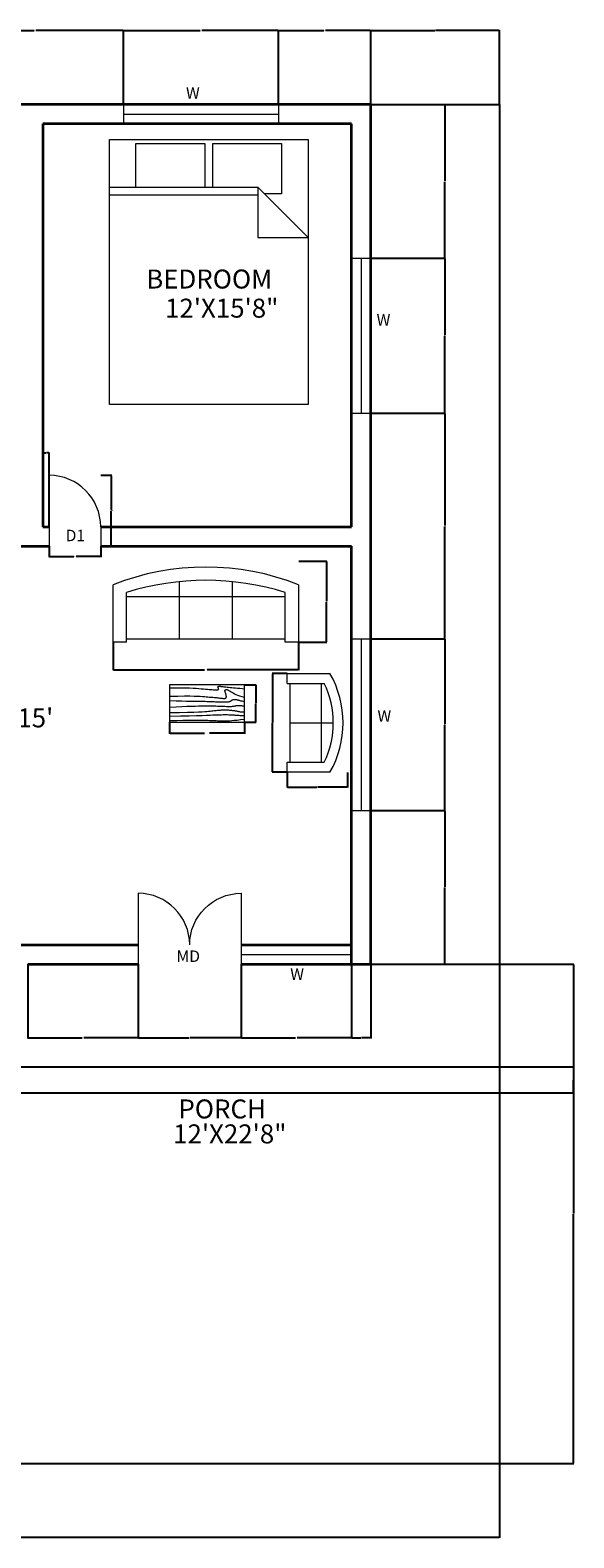
# Model space of a CAD drawing. Units: feet. Extents: x 1508 to 2265, y 1718 to 2421.
# Tile 4 of 4: x 2012 to 2265, y 1718 to 2421. Entities that reach past the tile are written whole.
import ezdxf

# ---------------------------------------------------------------- set-up
doc = ezdxf.new("R2010")
doc.units = ezdxf.units.FT
for name, color, linetype, lineweight in [('A-ANNO-DIMS', 2, 'Continuous', 18), ('A-ANNO-TEXT', 3, 'Continuous', 13), ('A-AREA-IDEN', 7, 'Continuous', 18), ('A-DOOR', 3, 'Continuous', 18), ('A-FURN', 8, 'Continuous', 18), ('A-GLAZ', 4, 'Continuous', 18), ('A-WALL', 7, 'Continuous', 35), ('C-PROP', 7, 'Continuous', 25)]:
    doc.layers.add(name, color=color, linetype=linetype, lineweight=lineweight)
doc.styles.get("Standard").update_dxf_attribs({"font": 'arial.ttf'})
doc.dimstyles.get("Standard").update_dxf_attribs({"dimtxt": 0.18, "dimasz": 0.18, "dimexe": 0.18, "dimexo": 0.0625, "dimgap": 0.09, "dimtad": 0, "dimtih": 1, "dimtoh": 1, "dimdec": 4, "dimzin": 0, "dimdsep": 46, "dimtxsty": 'Standard', "dimcen": 0.09, "dimadec": 0, "dimazin": 0, "dimtfac": 1, "dimtdec": 4, "dimtofl": 0, "dimtmove": 0, "dimatfit": 3, "dimfxl": 1, "dimtolj": 1, "dimtzin": 0, "dimarcsym": 0})

# ---------------------------------------------------------------- blocks, each defined once
blk = doc.blocks.new('Bed - Queen')
for p, q in [((0, -80.00003), (0, 0)), ((0, 0), (59.99999, 0)), ((59.99999, 0), (59.99999, -80.00003)), ((7.99999, -1.2), (28.79998, -1.2)), ((7.99999, -14.4), (7.99999, -1.2)), ((28.79998, -1.2), (28.79998, -14.4)), ((31.19999, -1.2), (51.99999, -1.2)), ((31.19999, -14.4), (31.19999, -1.2)), ((51.99999, -1.2), (51.99999, -16.4)), ((0, -14.4), (44.8, -14.4)), ((44.8, -16.8), (0, -16.8)), ((59.99999, -29.6), (44.8, -14.4)), ((44.8, -14.4), (44.8, -29.6)), ((51.99999, -16.4), (46.79936, -16.4)), ((44.8, -29.6), (59.99999, -29.6)), ((59.99999, -80.00003), (0, -80.00003))]:
    blk.add_line(p, q)
blk = doc.blocks.new('Sofa - Roundback 7 ft.')
for p, q in [((-12.00002, -32.4421), (-12.00003, -6.5971)), ((11.99997, -32.4421), (11.99998, -6.5971)), ((-36.000027, -34), (-36.000027, -11.4696)), ((-35.999844, -13.3819), (35.9998, -13.3819)), ((35.99998, -34), (35.99998, -11.4696)), ((-36.000027, -32.4421), (35.99998, -32.4421))]:
    blk.add_line(p, q)
for points in [[(-36.000027, -34), (-42.000027, -34), (-42.000027, -8)], [(41.99998, -8), (41.99998, -34), (35.99998, -34)]]:
    blk.add_lwpolyline(points)
for centre, radius, start, end in [((0, -114.25), 114.25, 68.43141, 111.5686), ((-0.00001, -127.1968), 121.1968, 72.72033, 107.2797)]:
    blk.add_arc(centre, radius, start, end)
blk = doc.blocks.new('Sofa - Roundback Loveseat 5 ft.')
for p, q in [((0, -32.44198), (0, -5.99998)), ((-24, -33.99998), (-24, -11.46958)), ((-23.9998, -13.38178), (23.99986, -13.38178)), ((24.00004, -33.99998), (24.00004, -11.46958)), ((-24, -32.44198), (24.00004, -32.44198))]:
    blk.add_line(p, q)
for points in [[(-24, -33.99998), (-30, -33.99998), (-30, -7.99998)], [(30.00004, -7.99998), (30.00004, -33.99998), (24.00004, -33.99998)]]:
    blk.add_lwpolyline(points)
for centre, radius, start, end in [((0, -60.24998), 60.24998, 60.13715, 119.8628), ((0, -61.38438), 55.38444, 64.32083, 115.6792)]:
    blk.add_arc(centre, radius, start, end)
blk = doc.blocks.new('Table - Rectangular Woodgrain 60 x 30 in.')
for p, q in [((0, 0), (0, -30)), ((60, 0), (0, 0)), ((60, -30), (60, 0)), ((0, -30), (60, -30))]:
    blk.add_line(p, q)
for points in [[(0, -2.4), (4.8155, -2.418), (9.0302, -2.4688), (12.709, -2.5477), (15.9167, -2.65), (18.7181, -2.7711), (21.1781, -2.9063), (23.3616, -3.0508), (25.3333, -3.2), (27.1477, -3.3495), (28.8172, -3.4958), (30.3437, -3.636), (31.7291, -3.7667), (32.9756, -3.8849), (34.0849, -3.9875), (35.059, -4.0714), (35.9, -4.1334), (36.6114, -4.1711), (37.2041, -4.1854), (37.6906, -4.1779), (38.0833, -4.15), (38.3948, -4.1034), (38.6375, -4.0396), (38.8239, -3.9602), (38.9666, -3.8667), (39.0764, -3.7608), (39.1573, -3.6448), (39.2116, -3.521), (39.2416, -3.3917), (39.2498, -3.2593), (39.2385, -3.1261), (39.21, -2.9944), (39.1666, -2.8667), (39.111, -2.7447), (39.0468, -2.6281), (38.978, -2.5163), (38.9083, -2.4083), (38.8418, -2.3035), (38.7823, -2.201), (38.7337, -2.1001), (38.7, -2), (38.6844, -1.9003), (38.6875, -1.8021), (38.7094, -1.707), (38.75, -1.6167), (38.8094, -1.5326), (38.8875, -1.4563), (38.9844, -1.3893), (39.1, -1.3333), (39.2351, -1.2896), (39.3937, -1.2583), (39.5804, -1.2396), (39.8, -1.2333), (40.057, -1.2396), (40.3562, -1.2583), (40.7023, -1.2896), (41.1, -1.3333), (41.5547, -1.3895), (42.0755, -1.4573), (42.6721, -1.5361), (43.3542, -1.625), (44.1316, -1.7233), (45.014, -1.8302), (46.0114, -1.9449), (47.1333, -2.0667), (48.3862, -2.1947), (49.7625, -2.3281), (51.2513, -2.4663), (52.8416, -2.6083), (54.5226, -2.7535), (56.2833, -2.9011), (58.1127, -3.0501), (60, -3.2)], [(0, -9.2), (6.5759, -9.0858), (11.9385, -9.0365), (16.2527, -9.0418), (19.6833, -9.0917), (22.3952, -9.1759), (24.5531, -9.2844), (26.322, -9.4069), (27.8666, -9.5333), (29.3241, -9.6553), (30.7203, -9.7719), (32.0532, -9.8837), (33.3208, -9.9917), (34.5213, -10.0965), (35.6526, -10.199), (36.7128, -10.2999), (37.7, -10.4), (38.6129, -10.4996), (39.4531, -10.5969), (40.223, -10.6895), (40.925, -10.775), (41.5613, -10.8512), (42.1344, -10.9156), (42.6465, -10.966), (43.1, -11), (43.4976, -11.0158), (43.8437, -11.0136), (44.143, -10.9942), (44.4, -10.9583), (44.6195, -10.9069), (44.8062, -10.8406), (44.9648, -10.7603), (45.1, -10.6667), (45.2155, -10.5598), (45.3114, -10.4365), (45.3871, -10.2929), (45.4416, -10.125), (45.4743, -9.929), (45.4844, -9.7011), (45.4709, -9.4371), (45.4333, -9.1333), (45.3716, -8.7883), (45.2896, -8.4104), (45.1919, -8.0107), (45.0833, -7.6), (44.9685, -7.1893), (44.8521, -6.7896), (44.7388, -6.4117), (44.6333, -6.0667), (44.54, -5.7628), (44.4614, -5.4979), (44.4001, -5.2675), (44.3583, -5.0667), (44.3384, -4.8909), (44.3427, -4.7354), (44.3736, -4.5956), (44.4333, -4.4667), (44.5236, -4.3453), (44.6427, -4.2333), (44.7884, -4.1339), (44.9583, -4.05), (45.1501, -3.9849), (45.3614, -3.9417), (45.59, -3.9234), (45.8333, -3.9333), (46.0915, -3.9749), (46.3734, -4.0531), (46.6906, -4.1736), (47.0542, -4.3417), (47.4756, -4.5629), (47.9661, -4.8427), (48.5372, -5.1866), (49.2, -5.6), (49.9676, -6.0844), (50.8594, -6.625), (51.8965, -7.2031), (53.1, -7.8), (54.491, -8.3969), (56.0906, -8.975), (57.9199, -9.5156), (60, -10)], [(0, -12.8), (5.1847, -12.9322), (9.6213, -13.0323), (13.3963, -13.1059), (16.5958, -13.1583), (19.3063, -13.1952), (21.614, -13.2219), (23.6054, -13.2439), (25.3666, -13.2667), (26.9728, -13.2947), (28.4531, -13.3281), (29.8256, -13.3663), (31.1083, -13.4083), (32.3191, -13.4535), (33.476, -13.501), (34.597, -13.5501), (35.7, -13.6), (36.7984, -13.6497), (37.8875, -13.6979), (38.9578, -13.743), (40, -13.7833), (41.0047, -13.8174), (41.9625, -13.8438), (42.864, -13.8607), (43.7, -13.8667), (44.4631, -13.8604), (45.1552, -13.8417), (45.7801, -13.8104), (46.3416, -13.7667), (46.8439, -13.7104), (47.2906, -13.6417), (47.6858, -13.5604), (48.0333, -13.4667), (48.3375, -13.3608), (48.6042, -13.2448), (48.8396, -13.121), (49.05, -12.9917), (49.2417, -12.8593), (49.4208, -12.7261), (49.5937, -12.5944), (49.7667, -12.4667), (49.9452, -12.3451), (50.1323, -12.2313), (50.3303, -12.1268), (50.5416, -12.0333), (50.7686, -11.9524), (51.0135, -11.8854), (51.2788, -11.8341), (51.5666, -11.8), (51.8785, -11.7843), (52.2116, -11.7865), (52.562, -11.8059), (52.926, -11.8417), (53.2998, -11.8931), (53.6795, -11.9594), (54.0614, -12.0397), (54.4416, -12.1333), (54.8223, -12.2401), (55.2293, -12.3625), (55.6942, -12.5037), (56.2489, -12.6667), (56.9251, -12.8547), (57.7545, -13.0708), (58.7689, -13.3182), (60, -13.6)], [(0, -18), (5.124, -17.7273), (9.6609, -17.5057), (13.6705, -17.3303), (17.2125, -17.1958), (20.3467, -17.0973), (23.1328, -17.0297), (25.6307, -16.9878), (27.9, -16.9667), (29.9928, -16.9617), (31.9302, -16.9703), (33.7254, -16.9907), (35.3917, -17.0208), (36.9423, -17.0588), (38.3906, -17.1026), (39.7499, -17.1503), (41.0333, -17.2), (42.2519, -17.2496), (43.4073, -17.2969), (44.4986, -17.3395), (45.525, -17.375), (46.4858, -17.4012), (47.3802, -17.4156), (48.2074, -17.416), (48.9667, -17.4), (49.6583, -17.3662), (50.2872, -17.3167), (50.8595, -17.2547), (51.3812, -17.1833), (51.8584, -17.1057), (52.2971, -17.025), (52.7034, -16.9443), (53.0833, -16.8667), (53.443, -16.7951), (53.789, -16.7313), (54.128, -16.6768), (54.4666, -16.6334), (54.8115, -16.6024), (55.1693, -16.5854), (55.5465, -16.5841), (55.95, -16.6), (56.3828, -16.6337), (56.8346, -16.6823), (57.2915, -16.7418), (57.7396, -16.8084), (58.165, -16.878), (58.5539, -16.9469), (58.8924, -17.0111), (59.1666, -17.0667), (59.3679, -17.1107), (59.5078, -17.1438), (59.6032, -17.1675), (59.6708, -17.1833), (59.7275, -17.193), (59.7901, -17.1979), (59.8753, -17.1998), (60, -17.2)], [(0, -22.4), (8.0098, -22.2501), (14.4094, -22.1011), (19.4168, -21.9535), (23.25, -21.8083), (26.1269, -21.6663), (28.2656, -21.5281), (29.884, -21.3947), (31.2, -21.2667), (32.3967, -21.1448), (33.5172, -21.0292), (34.5697, -20.9198), (35.5625, -20.8167), (36.5037, -20.7198), (37.4015, -20.6292), (38.2642, -20.5448), (39.1, -20.4667), (39.9164, -20.3951), (40.7187, -20.3313), (41.5117, -20.2768), (42.3, -20.2333), (43.0883, -20.2024), (43.8812, -20.1854), (44.6836, -20.1841), (45.5, -20.2), (46.3328, -20.234), (47.1747, -20.2844), (48.0163, -20.3488), (48.8479, -20.425), (49.66, -20.5106), (50.4429, -20.6031), (51.1872, -20.7004), (51.8833, -20.8), (52.5246, -20.8999), (53.1166, -20.9995), (53.6681, -21.0983), (54.1875, -21.1958), (54.6834, -21.2919), (55.1646, -21.3859), (55.6394, -21.4777), (56.1167, -21.5667), (56.6028, -21.6515), (57.0961, -21.7266), (57.5929, -21.7852), (58.0896, -21.8208), (58.5823, -21.8268), (59.0674, -21.7964), (59.5412, -21.723), (60, -21.6)], [(0, -25.2), (8.6355, -25.0504), (15.7026, -24.9031), (21.4049, -24.7606), (25.9458, -24.625), (29.529, -24.4988), (32.3578, -24.3844), (34.6359, -24.284), (36.5667, -24.2), (38.3213, -24.1341), (39.9417, -24.0854), (41.437, -24.0523), (42.8167, -24.0333), (44.0901, -24.0268), (45.2667, -24.0313), (46.3557, -24.0451), (47.3667, -24.0667), (48.309, -24.0947), (49.1928, -24.1287), (50.0284, -24.168), (50.826, -24.2125), (51.5959, -24.2617), (52.3483, -24.3151), (53.0935, -24.3725), (53.8417, -24.4334), (54.6009, -24.497), (55.3699, -24.561), (56.1454, -24.6226), (56.9239, -24.6792), (57.7021, -24.7279), (58.4764, -24.7662), (59.2435, -24.7911), (60, -24.8)], [(0, -28.8), (5.6867, -28.6681), (10.45, -28.5698), (14.407, -28.5012), (17.675, -28.4584), (20.3711, -28.4374), (22.6125, -28.4344), (24.5164, -28.4455), (26.2, -28.4667), (27.762, -28.4947), (29.2276, -28.5281), (30.6033, -28.5663), (31.8958, -28.6084), (33.1118, -28.6535), (34.2578, -28.7011), (35.3405, -28.7501), (36.3666, -28.8), (37.3443, -28.8497), (38.288, -28.8974), (39.2137, -28.9412), (40.1375, -28.9792), (41.0753, -29.0093), (42.0432, -29.0297), (43.0572, -29.0384), (44.1333, -29.0333), (45.2936, -29.0114), (46.5843, -28.9641), (48.0579, -28.8816), (49.7666, -28.7542), (51.7629, -28.5721), (54.0989, -28.3255), (56.8272, -28.0048), (60, -27.6)]]:
    blk.add_lwpolyline(points)
blk = doc.blocks.new('DOOR-LEAF-24')
blk.add_line((0, 33), (0, 0))
blk.add_arc((0, 9), 24, 0, 90)
blk = doc.blocks.new('*D11')
at = {"layer": 'A-ANNO-DIMS', "color": 0, "lineweight": -2, "transparency": 16777216}
for p, q in [((2044.87, 2213.26), (2049.93, 2213.26)), ((2049.75, 2213.08), (2049.75, 2196.94)), ((2049.75, 2180.44), (2049.75, 2196.58)), ((2044.87, 2180.26), (2049.93, 2180.26))]:
    blk.add_line(p, q, dxfattribs=at)
at = {"layer": 'A-ANNO-DIMS', "color": 0, "transparency": 16777216}
for points in [[(2049.72, 2213.08), (2049.78, 2213.08), (2049.75, 2213.26)], [(2049.72, 2180.44), (2049.78, 2180.44), (2049.75, 2180.26)]]:
    blk.add_solid(points, dxfattribs=at)
at = {"layer": 'Defpoints', "color": 0, "transparency": 16777216}
for p in [(2044.8, 2213.26), (2049.75, 2213.26), (2044.8, 2180.26)]:
    blk.add_point(p, dxfattribs=at)
at = {"layer": 'A-ANNO-DIMS', "color": 0, "transparency": 16777216, "insert": (2049.75, 2196.76), "char_height": 0.18, "attachment_point": 5}
blk.add_mtext('\\A1;D1 SWING 33 TYP.', dxfattribs=at)
blk = doc.blocks.new('*D12')
at = {"layer": 'A-ANNO-DIMS', "color": 0, "lineweight": -2, "transparency": 16777216}
for p, q in [((2020.8, 2180.2), (2020.8, 2175.13)), ((2020.98, 2175.31), (2032.28, 2175.31)), ((2044.62, 2175.31), (2033.33, 2175.31)), ((2044.8, 2180.2), (2044.8, 2175.13))]:
    blk.add_line(p, q, dxfattribs=at)
at = {"layer": 'A-ANNO-DIMS', "color": 0, "transparency": 16777216}
for points in [[(2020.98, 2175.34), (2020.98, 2175.28), (2020.8, 2175.31)], [(2044.62, 2175.34), (2044.62, 2175.28), (2044.8, 2175.31)]]:
    blk.add_solid(points, dxfattribs=at)
at = {"layer": 'Defpoints', "color": 0, "transparency": 16777216}
for p in [(2020.8, 2180.26), (2044.8, 2180.26), (2044.8, 2175.31)]:
    blk.add_point(p, dxfattribs=at)
at = {"layer": 'A-ANNO-DIMS', "color": 0, "transparency": 16777216, "insert": (2032.8, 2175.31), "char_height": 0.18, "attachment_point": 5}
blk.add_mtext('\\A1;24 TYP.', dxfattribs=at)
blk = doc.blocks.new('*D19')
at = {"layer": 'A-ANNO-DIMS', "color": 0, "lineweight": -2, "transparency": 16777216}
for p, q in [((2050.62, 2135.39), (2050.62, 2122.3)), ((2137.08, 2135.39), (2137.08, 2122.3)), ((2050.8, 2122.48), (2093.25, 2122.48)), ((2136.9, 2122.48), (2094.45, 2122.48))]:
    blk.add_line(p, q, dxfattribs=at)
at = {"layer": 'A-ANNO-DIMS', "color": 0, "transparency": 16777216}
for points in [[(2050.8, 2122.51), (2050.8, 2122.45), (2050.62, 2122.48)], [(2136.9, 2122.51), (2136.9, 2122.45), (2137.08, 2122.48)]]:
    blk.add_solid(points, dxfattribs=at)
at = {"layer": 'Defpoints', "color": 0, "transparency": 16777216}
for p in [(2050.62, 2135.45), (2137.08, 2135.45), (2137.08, 2122.48)]:
    blk.add_point(p, dxfattribs=at)
at = {"layer": 'A-ANNO-DIMS', "color": 0, "transparency": 16777216, "insert": (2093.85, 2122.48), "char_height": 0.18, "attachment_point": 5}
blk.add_mtext('\\A1;SOFA 86', dxfattribs=at)
blk = doc.blocks.new('*D20')
at = {"layer": 'A-ANNO-DIMS', "color": 0, "lineweight": -2, "transparency": 16777216}
for p, q in [((2137.14, 2173.19), (2150.23, 2173.19)), ((2150.05, 2173.01), (2150.05, 2154.5)), ((2150.05, 2135.63), (2150.05, 2154.14)), ((2137.14, 2135.45), (2150.23, 2135.45))]:
    blk.add_line(p, q, dxfattribs=at)
at = {"layer": 'A-ANNO-DIMS', "color": 0, "transparency": 16777216}
for points in [[(2150.02, 2173.01), (2150.08, 2173.01), (2150.05, 2173.19)], [(2150.02, 2135.63), (2150.08, 2135.63), (2150.05, 2135.45)]]:
    blk.add_solid(points, dxfattribs=at)
at = {"layer": 'Defpoints', "color": 0, "transparency": 16777216}
for p in [(2137.08, 2173.19), (2150.05, 2173.19), (2137.08, 2135.45)]:
    blk.add_point(p, dxfattribs=at)
at = {"layer": 'A-ANNO-DIMS', "color": 0, "transparency": 16777216, "insert": (2150.05, 2154.32), "char_height": 0.18, "attachment_point": 5}
blk.add_mtext('\\A1;38', dxfattribs=at)
blk = doc.blocks.new('*D21')
at = {"layer": 'A-ANNO-DIMS', "color": 0, "lineweight": -2, "transparency": 16777216}
for p, q in [((2131.73, 2120.8), (2124.71, 2120.8)), ((2124.89, 2120.62), (2124.89, 2097.97)), ((2124.89, 2074.95), (2124.89, 2097.6)), ((2131.73, 2074.77), (2124.71, 2074.77))]:
    blk.add_line(p, q, dxfattribs=at)
at = {"layer": 'A-ANNO-DIMS', "color": 0, "transparency": 16777216}
for points in [[(2124.86, 2120.62), (2124.92, 2120.62), (2124.89, 2120.8)], [(2124.86, 2074.95), (2124.92, 2074.95), (2124.89, 2074.77)]]:
    blk.add_solid(points, dxfattribs=at)
at = {"layer": 'Defpoints', "color": 0, "transparency": 16777216}
for p in [(2131.79, 2120.8), (2124.89, 2074.77), (2131.79, 2074.77)]:
    blk.add_point(p, dxfattribs=at)
at = {"layer": 'A-ANNO-DIMS', "color": 0, "transparency": 16777216, "insert": (2124.89, 2097.78), "char_height": 0.18, "attachment_point": 5}
blk.add_mtext('\\A1;LOVESEAT 46', dxfattribs=at)
blk = doc.blocks.new('*D22')
at = {"layer": 'A-ANNO-DIMS', "color": 0, "lineweight": -2, "transparency": 16777216}
for p, q in [((2131.79, 2074.7), (2131.79, 2067.68)), ((2131.97, 2067.86), (2145.64, 2067.86)), ((2159.74, 2067.86), (2146.08, 2067.86)), ((2159.92, 2074.7), (2159.92, 2067.68))]:
    blk.add_line(p, q, dxfattribs=at)
at = {"layer": 'A-ANNO-DIMS', "color": 0, "transparency": 16777216}
for points in [[(2131.97, 2067.89), (2131.97, 2067.83), (2131.79, 2067.86)], [(2159.74, 2067.89), (2159.74, 2067.83), (2159.92, 2067.86)]]:
    blk.add_solid(points, dxfattribs=at)
at = {"layer": 'Defpoints', "color": 0, "transparency": 16777216}
for p in [(2131.79, 2074.77), (2159.92, 2074.77), (2159.92, 2067.86)]:
    blk.add_point(p, dxfattribs=at)
at = {"layer": 'A-ANNO-DIMS', "color": 0, "transparency": 16777216, "insert": (2145.86, 2067.86), "char_height": 0.18, "attachment_point": 5}
blk.add_mtext('\\A1;28', dxfattribs=at)
blk = doc.blocks.new('*D23')
at = {"layer": 'A-ANNO-DIMS', "color": 0, "lineweight": -2, "transparency": 16777216}
for p, q in [((2076.97, 2098.08), (2076.97, 2092.73)), ((2111.87, 2098.08), (2111.87, 2092.73)), ((2077.15, 2092.91), (2093.22, 2092.91)), ((2111.69, 2092.91), (2095.61, 2092.91))]:
    blk.add_line(p, q, dxfattribs=at)
at = {"layer": 'A-ANNO-DIMS', "color": 0, "transparency": 16777216}
for points in [[(2077.15, 2092.94), (2077.15, 2092.88), (2076.97, 2092.91)], [(2111.69, 2092.94), (2111.69, 2092.88), (2111.87, 2092.91)]]:
    blk.add_solid(points, dxfattribs=at)
at = {"layer": 'Defpoints', "color": 0, "transparency": 16777216}
for p in [(2076.97, 2098.14), (2111.87, 2098.14), (2111.87, 2092.91)]:
    blk.add_point(p, dxfattribs=at)
at = {"layer": 'A-ANNO-DIMS', "color": 0, "transparency": 16777216, "insert": (2094.42, 2092.91), "char_height": 0.18, "attachment_point": 5}
blk.add_mtext('\\A1;COFFEE TABLE 35', dxfattribs=at)
blk = doc.blocks.new('*D24')
at = {"layer": 'A-ANNO-DIMS', "color": 0, "lineweight": -2, "transparency": 16777216}
for p, q in [((2111.93, 2115.59), (2117.28, 2115.59)), ((2117.1, 2115.41), (2117.1, 2107.04)), ((2117.1, 2098.32), (2117.1, 2106.68)), ((2111.93, 2098.14), (2117.28, 2098.14))]:
    blk.add_line(p, q, dxfattribs=at)
at = {"layer": 'A-ANNO-DIMS', "color": 0, "transparency": 16777216}
for points in [[(2117.07, 2115.41), (2117.13, 2115.41), (2117.1, 2115.59)], [(2117.07, 2098.32), (2117.13, 2098.32), (2117.1, 2098.14)]]:
    blk.add_solid(points, dxfattribs=at)
at = {"layer": 'Defpoints', "color": 0, "transparency": 16777216}
for p in [(2111.87, 2115.59), (2117.1, 2115.59), (2111.87, 2098.14)]:
    blk.add_point(p, dxfattribs=at)
at = {"layer": 'A-ANNO-DIMS', "color": 0, "transparency": 16777216, "insert": (2117.1, 2106.86), "char_height": 0.18, "attachment_point": 5}
blk.add_mtext('\\A1;17', dxfattribs=at)
blk = doc.blocks.new('*D31')
at = {"layer": 'A-ANNO-DIMS', "color": 0, "lineweight": -2, "transparency": 16777216}
for p, q in [((1542.8, 1752.2), (1542.8, 1717.61)), ((2230.8, 1752.2), (2230.8, 1717.61)), ((1542.98, 1717.79), (1886.52, 1717.79)), ((2230.62, 1717.79), (1887.09, 1717.79))]:
    blk.add_line(p, q, dxfattribs=at)
at = {"layer": 'A-ANNO-DIMS', "color": 0, "transparency": 16777216}
for points in [[(1542.98, 1717.82), (1542.98, 1717.76), (1542.8, 1717.79)], [(2230.62, 1717.82), (2230.62, 1717.76), (2230.8, 1717.79)]]:
    blk.add_solid(points, dxfattribs=at)
at = {"layer": 'Defpoints', "color": 0, "transparency": 16777216}
for p in [(1542.8, 1752.26), (2230.8, 1752.26), (2230.8, 1717.79)]:
    blk.add_point(p, dxfattribs=at)
at = {"layer": 'A-ANNO-DIMS', "color": 0, "transparency": 16777216, "insert": (1886.8, 1717.79), "char_height": 0.18, "attachment_point": 5}
blk.add_mtext('\\A1;688', dxfattribs=at)
blk = doc.blocks.new('*D34')
at = {"layer": 'A-ANNO-DIMS', "color": 0, "lineweight": -2, "transparency": 16777216}
for p, q in [((2170.8, 2386.32), (2170.8, 2420.92)), ((2170.98, 2420.74), (2200.59, 2420.74)), ((2230.62, 2420.74), (2201.02, 2420.74)), ((2230.8, 2386.32), (2230.8, 2420.92))]:
    blk.add_line(p, q, dxfattribs=at)
at = {"layer": 'A-ANNO-DIMS', "color": 0, "transparency": 16777216}
for points in [[(2170.98, 2420.77), (2170.98, 2420.71), (2170.8, 2420.74)], [(2230.62, 2420.77), (2230.62, 2420.71), (2230.8, 2420.74)]]:
    blk.add_solid(points, dxfattribs=at)
at = {"layer": 'Defpoints', "color": 0, "transparency": 16777216}
for p in [(2230.8, 2420.74), (2170.8, 2386.26), (2230.8, 2386.26)]:
    blk.add_point(p, dxfattribs=at)
at = {"layer": 'A-ANNO-DIMS', "color": 0, "transparency": 16777216, "insert": (2200.8, 2420.74), "char_height": 0.18, "attachment_point": 5}
blk.add_mtext('\\A1;60', dxfattribs=at)
blk = doc.blocks.new('*D44')
at = {"layer": 'A-ANNO-DIMS', "color": 0, "lineweight": -2, "transparency": 16777216}
for p, q in [((1972.97, 2386.32), (1972.97, 2420.92)), ((1973.15, 2420.74), (2013.79, 2420.74)), ((2055.22, 2420.74), (2014.58, 2420.74)), ((2055.4, 2386.32), (2055.4, 2420.92))]:
    blk.add_line(p, q, dxfattribs=at)
at = {"layer": 'A-ANNO-DIMS', "color": 0, "transparency": 16777216}
for points in [[(1973.15, 2420.77), (1973.15, 2420.71), (1972.97, 2420.74)], [(2055.22, 2420.77), (2055.22, 2420.71), (2055.4, 2420.74)]]:
    blk.add_solid(points, dxfattribs=at)
at = {"layer": 'Defpoints', "color": 0, "transparency": 16777216}
for p in [(2055.4, 2420.74), (1972.97, 2386.26), (2055.4, 2386.26)]:
    blk.add_point(p, dxfattribs=at)
at = {"layer": 'A-ANNO-DIMS', "color": 0, "transparency": 16777216, "insert": (2014.19, 2420.74), "char_height": 0.18, "attachment_point": 5}
blk.add_mtext('\\A1;82.43', dxfattribs=at)
blk = doc.blocks.new('*D45')
at = {"layer": 'A-ANNO-DIMS', "color": 0, "lineweight": -2, "transparency": 16777216}
for p, q in [((2055.4, 2386.32), (2055.4, 2420.92)), ((2055.58, 2420.74), (2091.19, 2420.74)), ((2127.59, 2420.74), (2091.98, 2420.74)), ((2127.77, 2386.32), (2127.77, 2420.92))]:
    blk.add_line(p, q, dxfattribs=at)
at = {"layer": 'A-ANNO-DIMS', "color": 0, "transparency": 16777216}
for points in [[(2055.58, 2420.77), (2055.58, 2420.71), (2055.4, 2420.74)], [(2127.59, 2420.77), (2127.59, 2420.71), (2127.77, 2420.74)]]:
    blk.add_solid(points, dxfattribs=at)
at = {"layer": 'Defpoints', "color": 0, "transparency": 16777216}
for p in [(2127.77, 2420.74), (2055.4, 2386.26), (2127.77, 2386.26)]:
    blk.add_point(p, dxfattribs=at)
at = {"layer": 'A-ANNO-DIMS', "color": 0, "transparency": 16777216, "insert": (2091.59, 2420.74), "char_height": 0.18, "attachment_point": 5}
blk.add_mtext('\\A1;72.37', dxfattribs=at)
blk = doc.blocks.new('*D46')
at = {"layer": 'A-ANNO-DIMS', "color": 0, "lineweight": -2, "transparency": 16777216}
for p, q in [((2127.77, 2386.32), (2127.77, 2420.92)), ((2127.95, 2420.74), (2148.89, 2420.74)), ((2170.62, 2420.74), (2149.69, 2420.74)), ((2170.8, 2386.32), (2170.8, 2420.92))]:
    blk.add_line(p, q, dxfattribs=at)
at = {"layer": 'A-ANNO-DIMS', "color": 0, "transparency": 16777216}
for points in [[(2127.95, 2420.77), (2127.95, 2420.71), (2127.77, 2420.74)], [(2170.62, 2420.77), (2170.62, 2420.71), (2170.8, 2420.74)]]:
    blk.add_solid(points, dxfattribs=at)
at = {"layer": 'Defpoints', "color": 0, "transparency": 16777216}
for p in [(2170.8, 2420.74), (2127.77, 2386.26), (2170.8, 2386.26)]:
    blk.add_point(p, dxfattribs=at)
at = {"layer": 'A-ANNO-DIMS', "color": 0, "transparency": 16777216, "insert": (2149.29, 2420.74), "char_height": 0.18, "attachment_point": 5}
blk.add_mtext('\\A1;43.03', dxfattribs=at)
blk = doc.blocks.new('*D47')
at = {"layer": 'A-ANNO-DIMS', "color": 0, "lineweight": -2, "transparency": 16777216}
for p, q in [((2170.87, 1985.26), (2265.46, 1985.26)), ((2265.28, 1985.08), (2265.28, 1868.94)), ((2265.28, 1752.44), (2265.28, 1868.58)), ((2230.87, 1752.26), (2265.46, 1752.26))]:
    blk.add_line(p, q, dxfattribs=at)
at = {"layer": 'A-ANNO-DIMS', "color": 0, "transparency": 16777216}
for points in [[(2265.25, 1985.08), (2265.31, 1985.08), (2265.28, 1985.26)], [(2265.25, 1752.44), (2265.31, 1752.44), (2265.28, 1752.26)]]:
    blk.add_solid(points, dxfattribs=at)
at = {"layer": 'Defpoints', "color": 0, "transparency": 16777216}
for p in [(2170.8, 1985.26), (2265.28, 1985.26), (2230.8, 1752.26)]:
    blk.add_point(p, dxfattribs=at)
at = {"layer": 'A-ANNO-DIMS', "color": 0, "transparency": 16777216, "insert": (2265.28, 1868.76), "char_height": 0.18, "attachment_point": 5}
blk.add_mtext('\\A1;233', dxfattribs=at)
blk = doc.blocks.new('*D48')
at = {"layer": 'A-ANNO-DIMS', "color": 0, "lineweight": -2, "transparency": 16777216}
for p, q in [((2170.87, 2056.93), (2205.46, 2056.93)), ((2205.28, 2056.75), (2205.28, 2021.28)), ((2205.28, 1985.44), (2205.28, 2020.91)), ((2170.87, 1985.26), (2205.46, 1985.26))]:
    blk.add_line(p, q, dxfattribs=at)
at = {"layer": 'A-ANNO-DIMS', "color": 0, "transparency": 16777216}
for points in [[(2205.25, 2056.75), (2205.31, 2056.75), (2205.28, 2056.93)], [(2205.25, 1985.44), (2205.31, 1985.44), (2205.28, 1985.26)]]:
    blk.add_solid(points, dxfattribs=at)
at = {"layer": 'Defpoints', "color": 0, "transparency": 16777216}
for p in [(2170.8, 2056.93), (2170.8, 1985.26), (2205.28, 1985.26)]:
    blk.add_point(p, dxfattribs=at)
at = {"layer": 'A-ANNO-DIMS', "color": 0, "transparency": 16777216, "insert": (2205.28, 2021.1), "char_height": 0.18, "attachment_point": 5}
blk.add_mtext('\\A1;71.67', dxfattribs=at)
blk = doc.blocks.new('*D49')
at = {"layer": 'A-ANNO-DIMS', "color": 0, "lineweight": -2, "transparency": 16777216}
for p, q in [((2170.87, 2136.96), (2205.46, 2136.96)), ((2205.28, 2136.78), (2205.28, 2097.13)), ((2205.28, 2057.11), (2205.28, 2096.76)), ((2170.87, 2056.93), (2205.46, 2056.93))]:
    blk.add_line(p, q, dxfattribs=at)
at = {"layer": 'A-ANNO-DIMS', "color": 0, "transparency": 16777216}
for points in [[(2205.25, 2136.78), (2205.31, 2136.78), (2205.28, 2136.96)], [(2205.25, 2057.11), (2205.31, 2057.11), (2205.28, 2056.93)]]:
    blk.add_solid(points, dxfattribs=at)
at = {"layer": 'Defpoints', "color": 0, "transparency": 16777216}
for p in [(2170.8, 2136.96), (2170.8, 2056.93), (2205.28, 2056.93)]:
    blk.add_point(p, dxfattribs=at)
at = {"layer": 'A-ANNO-DIMS', "color": 0, "transparency": 16777216, "insert": (2205.28, 2096.94), "char_height": 0.18, "attachment_point": 5}
blk.add_mtext('\\A1;80.03', dxfattribs=at)
blk = doc.blocks.new('*D50')
at = {"layer": 'A-ANNO-DIMS', "color": 0, "lineweight": -2, "transparency": 16777216}
for p, q in [((2170.87, 2242.23), (2205.46, 2242.23)), ((2205.28, 2242.05), (2205.28, 2189.78)), ((2205.28, 2137.14), (2205.28, 2189.41)), ((2170.87, 2136.96), (2205.46, 2136.96))]:
    blk.add_line(p, q, dxfattribs=at)
at = {"layer": 'A-ANNO-DIMS', "color": 0, "transparency": 16777216}
for points in [[(2205.25, 2242.05), (2205.31, 2242.05), (2205.28, 2242.23)], [(2205.25, 2137.14), (2205.31, 2137.14), (2205.28, 2136.96)]]:
    blk.add_solid(points, dxfattribs=at)
at = {"layer": 'Defpoints', "color": 0, "transparency": 16777216}
for p in [(2170.8, 2242.23), (2170.8, 2136.96), (2205.28, 2136.96)]:
    blk.add_point(p, dxfattribs=at)
at = {"layer": 'A-ANNO-DIMS', "color": 0, "transparency": 16777216, "insert": (2205.28, 2189.6), "char_height": 0.18, "attachment_point": 5}
blk.add_mtext('\\A1;105.28', dxfattribs=at)
blk = doc.blocks.new('*D51')
at = {"layer": 'A-ANNO-DIMS', "color": 0, "lineweight": -2, "transparency": 16777216}
for p, q in [((2170.87, 2314.57), (2205.46, 2314.57)), ((2205.28, 2314.39), (2205.28, 2278.58)), ((2205.28, 2242.41), (2205.28, 2278.22)), ((2170.87, 2242.23), (2205.46, 2242.23))]:
    blk.add_line(p, q, dxfattribs=at)
at = {"layer": 'A-ANNO-DIMS', "color": 0, "transparency": 16777216}
for points in [[(2205.25, 2314.39), (2205.31, 2314.39), (2205.28, 2314.57)], [(2205.25, 2242.41), (2205.31, 2242.41), (2205.28, 2242.23)]]:
    blk.add_solid(points, dxfattribs=at)
at = {"layer": 'Defpoints', "color": 0, "transparency": 16777216}
for p in [(2170.8, 2314.57), (2170.8, 2242.23), (2205.28, 2242.23)]:
    blk.add_point(p, dxfattribs=at)
at = {"layer": 'A-ANNO-DIMS', "color": 0, "transparency": 16777216, "insert": (2205.28, 2278.4), "char_height": 0.18, "attachment_point": 5}
blk.add_mtext('\\A1;72.34', dxfattribs=at)
blk = doc.blocks.new('*D52')
at = {"layer": 'A-ANNO-DIMS', "color": 0, "lineweight": -2, "transparency": 16777216}
for p, q in [((2170.87, 2386.26), (2205.46, 2386.26)), ((2205.28, 2386.08), (2205.28, 2350.6)), ((2205.28, 2314.75), (2205.28, 2350.23)), ((2170.87, 2314.57), (2205.46, 2314.57))]:
    blk.add_line(p, q, dxfattribs=at)
at = {"layer": 'A-ANNO-DIMS', "color": 0, "transparency": 16777216}
for points in [[(2205.25, 2386.08), (2205.31, 2386.08), (2205.28, 2386.26)], [(2205.25, 2314.75), (2205.31, 2314.75), (2205.28, 2314.57)]]:
    blk.add_solid(points, dxfattribs=at)
at = {"layer": 'Defpoints', "color": 0, "transparency": 16777216}
for p in [(2170.8, 2386.26), (2170.8, 2314.57), (2205.28, 2314.57)]:
    blk.add_point(p, dxfattribs=at)
at = {"layer": 'A-ANNO-DIMS', "color": 0, "transparency": 16777216, "insert": (2205.28, 2350.42), "char_height": 0.18, "attachment_point": 5}
blk.add_mtext('\\A1;71.69', dxfattribs=at)
blk = doc.blocks.new('*D75')
at = {"layer": 'A-ANNO-DIMS', "color": 0, "lineweight": -2, "transparency": 16777216}
for p, q in [((2010.8, 1985.2), (2010.8, 1950.61)), ((2062.3, 1985.2), (2062.3, 1950.61)), ((2010.98, 1950.79), (2036.23, 1950.79)), ((2062.12, 1950.79), (2036.88, 1950.79))]:
    blk.add_line(p, q, dxfattribs=at)
at = {"layer": 'A-ANNO-DIMS', "color": 0, "transparency": 16777216}
for points in [[(2010.98, 1950.82), (2010.98, 1950.76), (2010.8, 1950.79)], [(2062.12, 1950.82), (2062.12, 1950.76), (2062.3, 1950.79)]]:
    blk.add_solid(points, dxfattribs=at)
at = {"layer": 'Defpoints', "color": 0, "transparency": 16777216}
for p in [(2010.8, 1985.26), (2062.3, 1985.26), (2010.8, 1950.79)]:
    blk.add_point(p, dxfattribs=at)
at = {"layer": 'A-ANNO-DIMS', "color": 0, "transparency": 16777216, "insert": (2036.55, 1950.79), "char_height": 0.18, "attachment_point": 5}
blk.add_mtext('\\A1;51.5', dxfattribs=at)
blk = doc.blocks.new('*D76')
at = {"layer": 'A-ANNO-DIMS', "color": 0, "lineweight": -2, "transparency": 16777216}
for p, q in [((2062.3, 1985.2), (2062.3, 1950.61)), ((2110.3, 1985.2), (2110.3, 1950.61)), ((2062.48, 1950.79), (2086.08, 1950.79)), ((2110.12, 1950.79), (2086.53, 1950.79))]:
    blk.add_line(p, q, dxfattribs=at)
at = {"layer": 'A-ANNO-DIMS', "color": 0, "transparency": 16777216}
for points in [[(2062.48, 1950.82), (2062.48, 1950.76), (2062.3, 1950.79)], [(2110.12, 1950.82), (2110.12, 1950.76), (2110.3, 1950.79)]]:
    blk.add_solid(points, dxfattribs=at)
at = {"layer": 'Defpoints', "color": 0, "transparency": 16777216}
for p in [(2062.3, 1985.26), (2110.3, 1985.26), (2062.3, 1950.79)]:
    blk.add_point(p, dxfattribs=at)
at = {"layer": 'A-ANNO-DIMS', "color": 0, "transparency": 16777216, "insert": (2086.3, 1950.79), "char_height": 0.18, "attachment_point": 5}
blk.add_mtext('\\A1;48', dxfattribs=at)
blk = doc.blocks.new('*D77')
at = {"layer": 'A-ANNO-DIMS', "color": 0, "lineweight": -2, "transparency": 16777216}
for p, q in [((2110.3, 1985.2), (2110.3, 1950.61)), ((2161.8, 1985.2), (2161.8, 1950.61)), ((2110.48, 1950.79), (2135.73, 1950.79)), ((2161.62, 1950.79), (2136.38, 1950.79))]:
    blk.add_line(p, q, dxfattribs=at)
at = {"layer": 'A-ANNO-DIMS', "color": 0, "transparency": 16777216}
for points in [[(2110.48, 1950.82), (2110.48, 1950.76), (2110.3, 1950.79)], [(2161.62, 1950.82), (2161.62, 1950.76), (2161.8, 1950.79)]]:
    blk.add_solid(points, dxfattribs=at)
at = {"layer": 'Defpoints', "color": 0, "transparency": 16777216}
for p in [(2110.3, 1985.26), (2161.8, 1985.26), (2110.3, 1950.79)]:
    blk.add_point(p, dxfattribs=at)
at = {"layer": 'A-ANNO-DIMS', "color": 0, "transparency": 16777216, "insert": (2136.05, 1950.79), "char_height": 0.18, "attachment_point": 5}
blk.add_mtext('\\A1;51.5', dxfattribs=at)
blk = doc.blocks.new('*D78')
at = {"layer": 'A-ANNO-DIMS', "color": 0, "lineweight": -2, "transparency": 16777216}
for p, q in [((2161.8, 1985.2), (2161.8, 1950.61)), ((2170.8, 1985.2), (2170.8, 1950.61)), ((2161.98, 1950.79), (2166.16, 1950.79)), ((2170.62, 1950.79), (2166.45, 1950.79))]:
    blk.add_line(p, q, dxfattribs=at)
at = {"layer": 'A-ANNO-DIMS', "color": 0, "transparency": 16777216}
for points in [[(2161.98, 1950.82), (2161.98, 1950.76), (2161.8, 1950.79)], [(2170.62, 1950.82), (2170.62, 1950.76), (2170.8, 1950.79)]]:
    blk.add_solid(points, dxfattribs=at)
at = {"layer": 'Defpoints', "color": 0, "transparency": 16777216}
for p in [(2161.8, 1985.26), (2170.8, 1985.26), (2161.8, 1950.79)]:
    blk.add_point(p, dxfattribs=at)
at = {"layer": 'A-ANNO-DIMS', "color": 0, "transparency": 16777216, "insert": (2166.3, 1950.79), "char_height": 0.18, "attachment_point": 5}
blk.add_mtext('\\A1;9', dxfattribs=at)
blk = doc.blocks.new('*D79')
at = {"layer": 'A-ANNO-DIMS', "color": 0, "lineweight": -2, "transparency": 16777216}
for p, q in [((1864.87, 1937.26), (2265.46, 1937.26)), ((2265.28, 1937.08), (2265.28, 1931.44)), ((2265.28, 1925.44), (2265.28, 1931.08)), ((1864.87, 1925.26), (2265.46, 1925.26))]:
    blk.add_line(p, q, dxfattribs=at)
at = {"layer": 'A-ANNO-DIMS', "color": 0, "transparency": 16777216}
for points in [[(2265.25, 1937.08), (2265.31, 1937.08), (2265.28, 1937.26)], [(2265.25, 1925.44), (2265.31, 1925.44), (2265.28, 1925.26)]]:
    blk.add_solid(points, dxfattribs=at)
at = {"layer": 'Defpoints', "color": 0, "transparency": 16777216}
for p in [(1864.8, 1937.26), (1864.8, 1925.26), (2265.28, 1925.26)]:
    blk.add_point(p, dxfattribs=at)
at = {"layer": 'A-ANNO-DIMS', "color": 0, "transparency": 16777216, "insert": (2265.28, 1931.26), "char_height": 0.18, "attachment_point": 5}
blk.add_mtext('\\A1;12', dxfattribs=at)
blk = doc.blocks.new('*D85')
at = {"layer": 'A-ANNO-DIMS', "color": 0, "lineweight": -2, "transparency": 16777216}
for p, q in [((2017.8, 2189.32), (2017.8, 2223.92)), ((2017.98, 2223.74), (2019.16, 2223.74)), ((2020.62, 2223.74), (2019.45, 2223.74)), ((2020.8, 2189.32), (2020.8, 2223.92))]:
    blk.add_line(p, q, dxfattribs=at)
at = {"layer": 'A-ANNO-DIMS', "color": 0, "transparency": 16777216}
for points in [[(2017.98, 2223.77), (2017.98, 2223.71), (2017.8, 2223.74)], [(2020.62, 2223.77), (2020.62, 2223.71), (2020.8, 2223.74)]]:
    blk.add_solid(points, dxfattribs=at)
at = {"layer": 'Defpoints', "color": 0, "transparency": 16777216}
for p in [(2020.8, 2223.74), (2017.8, 2189.26), (2020.8, 2189.26)]:
    blk.add_point(p, dxfattribs=at)
at = {"layer": 'A-ANNO-DIMS', "color": 0, "transparency": 16777216, "insert": (2019.3, 2223.74), "char_height": 0.18, "attachment_point": 5}
blk.add_mtext('\\A1;3', dxfattribs=at)

msp = doc.modelspace()

# ---------------------------------------------------------------- linework, layer by layer
at = {"layer": 'A-DOOR'}
msp.add_line((2044.8049, 2189.2608), (2044.8049, 2180.2608), dxfattribs=at)
at = {"layer": 'A-GLAZ'}
for p, q in [((2055.3983, 2386.2608), (2055.3983, 2377.2608)), ((2127.7719, 2386.2608), (2127.7719, 2377.2608)), ((2055.3983, 2381.7608), (2127.7719, 2381.7608)), ((2161.8049, 2314.5715), (2170.8049, 2314.5715)), ((2166.3049, 2314.5715), (2166.3049, 2242.2344)), ((2161.8049, 2242.2344), (2170.8049, 2242.2344)), ((2161.8049, 2136.9558), (2170.8049, 2136.9558)), ((2166.3049, 2136.9558), (2166.3049, 2056.9306)), ((2161.8049, 2056.9306), (2170.8049, 2056.9306)), ((2110.3049, 1989.7608), (2161.8049, 1989.7608))]:
    msp.add_line(p, q, dxfattribs=at)
at = {"layer": 'A-WALL'}
for p, q in [((2170.8049, 2386.2608), (1864.8049, 2386.2608)), ((2170.8049, 1985.2608), (2170.8049, 2386.2608)), ((2161.8049, 2377.2608), (2017.8049, 2377.2608)), ((2017.8049, 2377.2608), (2017.8049, 2189.2608)), ((2161.8049, 2189.2608), (2161.8049, 2377.2608)), ((2017.8049, 2189.2608), (2020.8049, 2189.2608)), ((2044.8049, 2189.2608), (2161.8049, 2189.2608)), ((1900.8049, 2180.2608), (2020.8049, 2180.2608)), ((2044.8049, 2180.2608), (2161.8049, 2180.2608)), ((2161.8049, 1985.2608), (2161.8049, 2180.2608)), ((2170.8049, 1985.2608), (2170.8049, 2180.2608)), ((2001.8049, 1994.2608), (2062.3049, 1994.2608)), ((2110.3049, 1994.2608), (2161.8049, 1994.2608)), ((2010.8049, 1985.2608), (2062.3049, 1985.2608)), ((2110.3049, 1985.2608), (2170.8049, 1985.2608))]:
    msp.add_line(p, q, dxfattribs=at)
at = {"layer": 'C-PROP'}
for p, q in [((2170.8049, 2386.2608), (2230.8049, 2386.2608)), ((2230.8049, 2386.2608), (2230.8049, 1753.015)), ((1611.8049, 1752.2608), (2230.8049, 1752.2608)), ((2230.8049, 1753.015), (2230.8049, 1752.2608))]:
    msp.add_line(p, q, dxfattribs=at)

# ---------------------------------------------------------------- block references
at = {"layer": 'A-DOOR'}
for p in [(2020.805, 2180.261), (2062.305, 1985.261)]:
    msp.add_blockref('DOOR-LEAF-24', p, dxfattribs=at)
at = {"layer": 'A-DOOR', "extrusion": (0, 0, -1), "zscale": -1}
msp.add_blockref('DOOR-LEAF-24', (-2110.3048, 1985.261), dxfattribs=at)
at = {"layer": 'A-FURN'}
for name, p, xscale, yscale, zscale in [('Bed - Queen', (2048.9065, 2369.8454), 1.544203597856591, 1.544203597856591, 1.544203597856591), ('Sofa - Roundback 7 ft.', (2093.8503, 2170.4435), 1.029239410836423, 1.029239410836423, 1.029239410836423), ('Table - Rectangular Woodgrain 60 x 30 in.', (2076.9696, 2115.5884), 0.5815987943461581, 0.5815987943461581, 0.5815987943461581)]:
    msp.add_blockref(name, p, dxfattribs=dict(at, xscale=xscale, yscale=yscale, zscale=zscale))
at = {"layer": 'A-FURN', "xscale": 0.7672187418824958, "yscale": 0.7672187418824958, "zscale": 0.7672187418824958, "rotation": 270}
msp.add_blockref('Sofa - Roundback Loveseat 5 ft.', (2157.8789, 2097.7834), dxfattribs=at)

# ---------------------------------------------------------------- texts
at = {"layer": 'A-ANNO-TEXT'}
for s, height, p in [('W', 5.3453, (2084.5843, 2388.94)), ('W', 5.3453, (2173.4957, 2283.0842)), ('D1', 5.34528, (2028.4578, 2182.5211)), ('W', 5.3453, (2173.8876, 2098.3235)), ('MD', 5.34528, (2080.1789, 1986.252)), ('W', 5.3453, (2133.214, 1977.8654))]:
    msp.add_text(s, height=height, dxfattribs=at).set_placement(p)
at = {"layer": 'A-AREA-IDEN'}
for s, p in [('BEDROOM', (2066.0397, 2300.3901)), ('12\'X15\'8"', (2074.8167, 2286.8036)), ('34\'4"X15\'', (1969.8225, 2095.6807)), ('PORCH', (2081.061, 1913.2532)), ('12\'X22\'8"', (2078.5889, 1901.607))]:
    msp.add_text(s, height=8.85057, dxfattribs=at).set_placement(p)

# ---------------------------------------------------------------- dimensions: what is measured, and where the dimension line sits
at = {"layer": 'A-ANNO-DIMS'}
for base, p1, p2, override, picture, middle in [((2055.3983, 2420.7358), (1972.9732, 2386.2608), (2055.3983, 2386.2608), {"dimdec": 2, "dimlfac": 1, "dimrnd": 0, "dimzin": 0, "dimdsep": 46, "dimlunit": 2}, '*D44', (2014.1857, 2420.7358)), ((2127.7719, 2420.7358), (2055.3983, 2386.2608), (2127.7719, 2386.2608), {"dimdec": 2, "dimlfac": 1, "dimrnd": 0, "dimzin": 0, "dimdsep": 46, "dimlunit": 2}, '*D45', (2091.5851, 2420.7358)), ((2170.8049, 2420.7358), (2127.7719, 2386.2608), (2170.8049, 2386.2608), {"dimdec": 2, "dimlfac": 1, "dimrnd": 0, "dimzin": 0, "dimdsep": 46, "dimlunit": 2}, '*D46', (2149.2884, 2420.7358)), ((2230.8049, 2420.7358), (2170.8049, 2386.2608), (2230.8049, 2386.2608), {"dimdec": 0, "dimlfac": 1, "dimrnd": 0, "dimzin": 0, "dimdsep": 46, "dimlunit": 2}, '*D34', (2200.8049, 2420.7358)), ((2020.8049, 2223.7358), (2017.8049, 2189.2608), (2020.8049, 2189.2608), {"dimdec": 0, "dimlfac": 1, "dimrnd": 0, "dimzin": 0, "dimdsep": 46, "dimlunit": 2}, '*D85', (2019.3049, 2223.7358)), ((2159.9248, 2067.8618), (2131.7935, 2074.7668), (2159.9248, 2074.7668), {"dimdec": 0, "dimlfac": 1, "dimrnd": 0, "dimzin": 0, "dimdsep": 46, "dimlunit": 2}, '*D22', (2145.8592, 2067.8618)), ((2230.8049, 1717.7858), (1542.8049, 1752.2608), (2230.8049, 1752.2608), {"dimdec": 0, "dimlfac": 1, "dimrnd": 0, "dimzin": 0, "dimdsep": 46, "dimlunit": 2}, '*D31', (1886.8049, 1717.7858))]:
    dim = msp.add_linear_dim(base=base, p1=p1, p2=p2, dimstyle='Standard', override=override, dxfattribs=at)
    dim.commit()
    dim.dimension.update_dxf_attribs({"geometry": picture, "text_midpoint": middle})
for base, p1, p2, angle, override, picture, middle in [((2205.2799, 2314.5715), (2170.8049, 2386.2608), (2170.8049, 2314.5715), 270, {"dimdec": 2, "dimlfac": 1, "dimrnd": 0, "dimzin": 0, "dimdsep": 46, "dimlunit": 2}, '*D52', (2205.2799, 2350.4161)), ((2205.2799, 2242.2344), (2170.8049, 2314.5715), (2170.8049, 2242.2344), 270, {"dimdec": 2, "dimlfac": 1, "dimrnd": 0, "dimzin": 0, "dimdsep": 46, "dimlunit": 2}, '*D51', (2205.2799, 2278.4029)), ((2205.2799, 2136.9558), (2170.8049, 2242.2344), (2170.8049, 2136.9558), 270, {"dimdec": 2, "dimlfac": 1, "dimrnd": 0, "dimzin": 0, "dimdsep": 46, "dimlunit": 2}, '*D50', (2205.2799, 2189.5951)), ((2150.0467, 2173.1881), (2137.0783, 2135.4493), (2137.0783, 2173.1881), 90, {"dimdec": 0, "dimlfac": 1, "dimrnd": 0, "dimzin": 0, "dimdsep": 46, "dimlunit": 2}, '*D20', (2150.0467, 2154.3187)), ((2205.2799, 2056.9306), (2170.8049, 2136.9558), (2170.8049, 2056.9306), 270, {"dimdec": 2, "dimlfac": 1, "dimrnd": 0, "dimzin": 0, "dimdsep": 46, "dimlunit": 2}, '*D49', (2205.2799, 2096.9432)), ((2117.0999, 2115.5884), (2111.8655, 2098.1404), (2111.8655, 2115.5884), 90, {"dimdec": 0, "dimlfac": 1, "dimrnd": 0, "dimzin": 0, "dimdsep": 46, "dimlunit": 2}, '*D24', (2117.0999, 2106.8644)), ((2205.2799, 1985.2608), (2170.8049, 2056.9306), (2170.8049, 1985.2608), 270, {"dimdec": 2, "dimlfac": 1, "dimrnd": 0, "dimzin": 0, "dimdsep": 46, "dimlunit": 2}, '*D48', (2205.2799, 2021.0957)), ((2010.8049, 1950.7858), (2062.3049, 1985.2608), (2010.8049, 1985.2608), 180, {"dimdec": 1, "dimlfac": 1, "dimrnd": 0, "dimzin": 0, "dimdsep": 46, "dimlunit": 2}, '*D75', (2036.5549, 1950.7858)), ((2062.3049, 1950.7858), (2110.3049, 1985.2608), (2062.3049, 1985.2608), 180, {"dimdec": 0, "dimlfac": 1, "dimrnd": 0, "dimzin": 0, "dimdsep": 46, "dimlunit": 2}, '*D76', (2086.3049, 1950.7858)), ((2110.3049, 1950.7858), (2161.8049, 1985.2608), (2110.3049, 1985.2608), 180, {"dimdec": 1, "dimlfac": 1, "dimrnd": 0, "dimzin": 0, "dimdsep": 46, "dimlunit": 2}, '*D77', (2136.0549, 1950.7858)), ((2161.8049, 1950.7858), (2170.8049, 1985.2608), (2161.8049, 1985.2608), 180, {"dimdec": 0, "dimlfac": 1, "dimrnd": 0, "dimzin": 0, "dimdsep": 46, "dimlunit": 2}, '*D78', (2166.3049, 1950.7858)), ((2265.2799, 1985.2608), (2230.8049, 1752.2608), (2170.8049, 1985.2608), 90, {"dimdec": 0, "dimlfac": 1, "dimrnd": 0, "dimzin": 0, "dimdsep": 46, "dimlunit": 2}, '*D47', (2265.2799, 1868.7608)), ((2265.2799, 1925.2608), (1864.8049, 1937.2608), (1864.8049, 1925.2608), 90, {"dimdec": 0, "dimlfac": 1, "dimrnd": 0, "dimzin": 0, "dimdsep": 46, "dimlunit": 2}, '*D79', (2265.2799, 1931.2608))]:
    dim = msp.add_linear_dim(base=base, p1=p1, p2=p2, angle=angle, dimstyle='Standard', override=override, dxfattribs=at)
    dim.commit()
    dim.dimension.update_dxf_attribs({"geometry": picture, "text_midpoint": middle})
for base, p1, p2, angle, text, picture, middle in [((2049.7549, 2213.2608), (2044.8049, 2180.2608), (2044.8049, 2213.2608), 90, 'D1 SWING <> TYP.', '*D11', (2049.7549, 2196.7608)), ((2124.8885, 2074.7668), (2131.7935, 2120.7999), (2131.7935, 2074.7668), 270, 'LOVESEAT <>', '*D21', (2124.8885, 2097.7834))]:
    dim = msp.add_linear_dim(base=base, p1=p1, p2=p2, angle=angle, text=text, dimstyle='Standard', override={"dimdec": 0, "dimlfac": 1, "dimrnd": 0, "dimzin": 0, "dimdsep": 46, "dimlunit": 2}, dxfattribs=at)
    dim.commit()
    dim.dimension.update_dxf_attribs({"geometry": picture, "text_midpoint": middle})
for base, p1, p2, text, picture, middle in [((2044.8049, 2175.3108), (2020.8049, 2180.2608), (2044.8049, 2180.2608), '<> TYP.', '*D12', (2032.8049, 2175.3108)), ((2137.0783, 2122.4809), (2050.6222, 2135.4493), (2137.0783, 2135.4493), 'SOFA <>', '*D19', (2093.8502, 2122.4809)), ((2111.8655, 2092.9061), (2076.9696, 2098.1404), (2111.8655, 2098.1404), 'COFFEE TABLE <>', '*D23', (2094.4175, 2092.9061))]:
    dim = msp.add_linear_dim(base=base, p1=p1, p2=p2, text=text, dimstyle='Standard', override={"dimdec": 0, "dimlfac": 1, "dimrnd": 0, "dimzin": 0, "dimdsep": 46, "dimlunit": 2}, dxfattribs=at)
    dim.commit()
    dim.dimension.update_dxf_attribs({"geometry": picture, "text_midpoint": middle})

doc.saveas('drawing.dxf')
